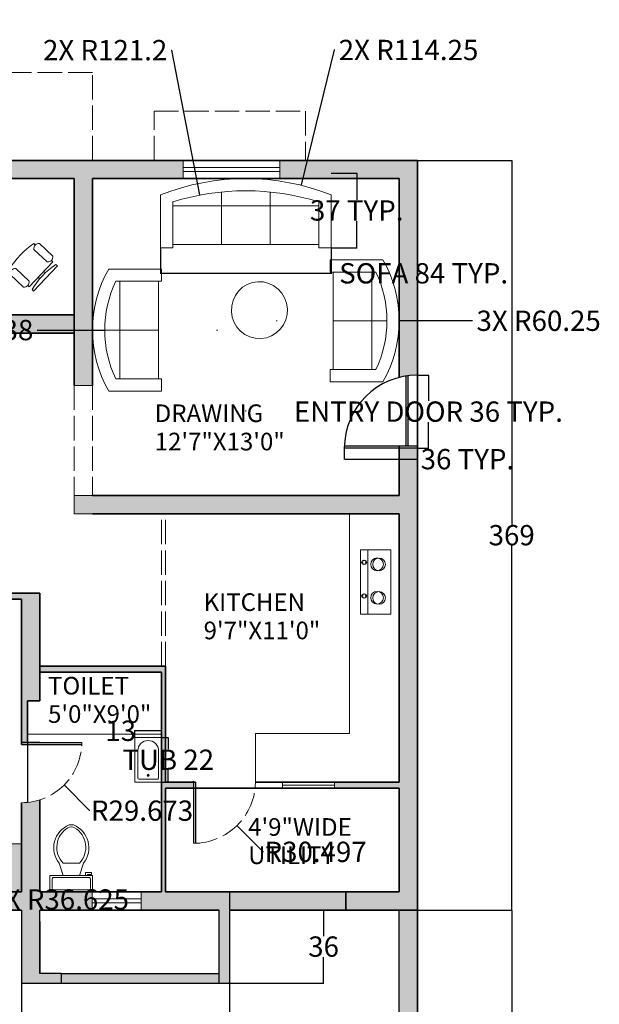
# Model space of a CAD drawing. Units: inches. Extents: x 215 to 969, y -612 to 418.
# Tile 8 of 8: x 684 to 969, y -93 to 391. Entities that reach past the tile are written whole.
import ezdxf

# ---------------------------------------------------------------- set-up
doc = ezdxf.new("R2010")
doc.units = ezdxf.units.IN
doc.header["$MEASUREMENT"] = 0
doc.linetypes.add('ACAD_ISO02W100', pattern=[15, 12, -3])
for name, color, linetype, lineweight in [('A-ANNO-DIMS', 2, 'Continuous', 18), ('A-AREA-IDEN', 7, 'Continuous', 18), ('A-DOOR', 3, 'Continuous', 25), ('A-DOOR-SWNG', 3, 'ACAD_ISO02W100', 13), ('A-EQPM', 8, 'Continuous', 18), ('A-FLOR-CASE', 9, 'Continuous', 18), ('A-FLOR-FIXT', 9, 'Continuous', 18), ('A-FLOR-OVHD', 8, 'ACAD_ISO02W100', 13), ('A-FLOR-SLAB', 7, 'Continuous', 25), ('A-FURN', 8, 'Continuous', 18), ('A-GLAZ', 4, 'Continuous', 18), ('A-WALL', 7, 'Continuous', 35), ('A-WALL-OVHD', 7, 'ACAD_ISO02W100', 18)]:
    doc.layers.add(name, color=color, linetype=linetype, lineweight=lineweight)
doc.layers.add('A-WALL-PATT', color=252, linetype='Continuous', lineweight=13, true_color=0x939598)
doc.styles.get("Standard").update_dxf_attribs({"font": 'arial.ttf'})
doc.dimstyles.get("Standard").update_dxf_attribs({"dimtxt": 10, "dimasz": 0.18, "dimexe": 0.18, "dimexo": 0.0625, "dimgap": 0.09, "dimtad": 0, "dimtih": 1, "dimtoh": 1, "dimdec": 0, "dimzin": 0, "dimdsep": 46, "dimlunit": 3, "dimtxsty": 'Standard', "dimcen": 0.09, "dimadec": 0, "dimazin": 0, "dimtfac": 1, "dimtdec": 0, "dimtofl": 0, "dimtmove": 0, "dimatfit": 3, "dimfxl": 1, "dimtolj": 1, "dimtzin": 0, "dimarcsym": 0})

# ---------------------------------------------------------------- blocks, each defined once
blk = doc.blocks.new('Sofa - Roundback 7 ft.')
for p, q in [((-12.00002, -32.4421), (-12.00003, -6.5971)), ((11.99997, -32.4421), (11.99998, -6.5971)), ((-36.000027, -34), (-36.000027, -11.4696)), ((-35.999844, -13.3819), (35.9998, -13.3819)), ((35.99998, -34), (35.99998, -11.4696)), ((-36.000027, -32.4421), (35.99998, -32.4421))]:
    blk.add_line(p, q)
for points in [[(-36.000027, -34), (-42.000027, -34), (-42.000027, -8)], [(41.99998, -8), (41.99998, -34), (35.99998, -34)]]:
    blk.add_lwpolyline(points)
for centre, radius, start, end in [((0, -114.25), 114.25, 68.43141, 111.5686), ((-0.00001, -127.1968), 121.1968, 72.72033, 107.2797)]:
    blk.add_arc(centre, radius, start, end)
blk = doc.blocks.new('Sofa - Roundback Loveseat 5 ft.')
for p, q in [((0, -32.44198), (0, -5.99998)), ((-24, -33.99998), (-24, -11.46958)), ((-23.9998, -13.38178), (23.99986, -13.38178)), ((24.00004, -33.99998), (24.00004, -11.46958)), ((-24, -32.44198), (24.00004, -32.44198))]:
    blk.add_line(p, q)
for points in [[(-24, -33.99998), (-30, -33.99998), (-30, -7.99998)], [(30.00004, -7.99998), (30.00004, -33.99998), (24.00004, -33.99998)]]:
    blk.add_lwpolyline(points)
for centre, radius, start, end in [((0, -60.24998), 60.24998, 60.13715, 119.8628), ((0, -61.38438), 55.38444, 64.32083, 115.6792)]:
    blk.add_arc(centre, radius, start, end)
blk = doc.blocks.new('Toilet - top')
for p, q in [((9.5, -6), (9.5, -2)), ((-10, -8.5), (-8, -8.5)), ((-10, -9.5), (-10, -8.5)), ((-7, -9.5), (-10, -9.5)), ((-8, -8.5), (-8, -8)), ((-7, -8), (-7, -9.5)), ((-4, -8), (-6, -14)), ((4, -8), (6, -14)), ((4, -14), (-4, -14))]:
    blk.add_line(p, q)
blk.add_lwpolyline([(10.5, -8), (10.5, 0), (-10.5, 0), (-10.5, -8)], close=True)
for points in [[(-9.5, -2), (-9.5, -6)], [(8.5, -1), (-8.5, -1)], [(-8.5, -7), (8.5, -7)]]:
    blk.add_lwpolyline(points)
for centre, radius, start, end in [((-8.62, -1.88), 0.884, 81.8699, 188.1301), ((8.62, -1.88), 0.884, 351.8699, 98.1301), ((-8.62, -6.12), 0.884, 171.8699, 278.1301), ((8.62, -6.12), 0.884, 261.8699, 8.1301), ((3.52, -21.58), 12.17, 141.4691, 247.9714), ((4.2, -21.82), 11.33, 136.3677, 238.9468), ((-3.52, -21.58), 12.17, 292.0284, 38.5307), ((-4.2, -21.82), 11.33, 301.053, 43.6321), ((0, -27.88), 4, 245.7318, 294.2682), ((0, -29), 4, 254.8605, 285.1395)]:
    blk.add_arc(centre, radius, start, end)
blk = doc.blocks.new('Bath Tub - 26 x 60 in.')
for p, q in [((8, -18), (10, -18)), ((9, -17), (9, -19))]:
    blk.add_line(p, q)
blk.add_lwpolyline([(0, -36), (0, 0), (60, 0), (60, -36)], close=True)
for points in [[(4, -30), (4, -6)], [(6, -4), (42, -4)], [(42, -32), (6, -32)]]:
    blk.add_lwpolyline(points)
for radius in [1.5, 1]:
    blk.add_circle((9, -18), radius)
for centre, radius, start, end in [((5.75, -5.75), 1.77, 81.8699, 188.1301), ((42, -18), 14, 270, 90), ((5.75, -30.25), 1.77, 171.8699, 278.1301)]:
    blk.add_arc(centre, radius, start, end)
blk = doc.blocks.new('Chair - Desk')
for p, q in [((-8.5, 0), (-8.5, -1)), ((-8.5, 0), (8.5, 0)), ((8.5, 0), (8.5, -1)), ((-8.5, -3), (-8.5, -4)), ((-8.5, -3), (8.5, -3)), ((-2, -3), (-2, -1.9355)), ((2, -1.9576), (2, -3)), ((8.5, -3), (8.5, -4)), ((-10.5, -5), (-10.5, -14)), ((-6.5, -14), (-6.5, -5)), ((6.5, -5), (6.5, -14)), ((10.5, -14), (10.5, -5)), ((-8.5, -15), (-8.5, -16)), ((8.5, -15), (8.5, -16))]:
    blk.add_line(p, q)
for centre, radius, start, end in [((-8.5, -6.5), 2.5, 36.8699, 143.1301), ((0, 34.625), 36.625, 256.5803, 283.4197), ((8.5, -6.5), 2.5, 36.8699, 143.1301), ((-8.5, -12.5), 2.5, 216.8699, 323.1301), ((8.5, -12.5), 2.5, 216.8699, 323.1301), ((0, 19.625), 36.625, 256.5803, 283.4197)]:
    blk.add_arc(centre, radius, start, end)
blk = doc.blocks.new('WINDOW-SHADE-75')
for p, q in [((0, 0), (0, 24.15)), ((0, 24.15), (74.66, 24.15)), ((74.66, 24.15), (74.66, 0))]:
    blk.add_line(p, q)
blk = doc.blocks.new('DOOR-ENTRY-36')
for p, q in [((36, 1), (0, 1)), ((36, 0), (0, 0))]:
    blk.add_line(p, q)
blk.add_arc((36, 0), 36, 90, 180)
blk = doc.blocks.new('WIN-FRAME-24B')
for p, q in [((0, 23.99), (9, 23.99)), ((3.5, 23.99), (3.5, 0)), ((5.5, 23.99), (5.5, 0)), ((9, 0), (0, 0)), ((4.5, 0), (9, 0))]:
    blk.add_line(p, q)
blk = doc.blocks.new('*D27')
at = {"layer": 'A-ANNO-DIMS', "color": 0, "lineweight": -2, "transparency": 16777216}
for p, q in [((753.42, 38.14), (756.82, 38.14)), ((756.64, 37.96), (756.64, 32.37)), ((756.64, 16.39), (756.64, 21.98)), ((753.42, 16.21), (756.82, 16.21))]:
    blk.add_line(p, q, dxfattribs=at)
at = {"layer": 'A-ANNO-DIMS', "color": 0, "transparency": 16777216}
for points in [[(756.61, 37.96), (756.67, 37.96), (756.64, 38.14)], [(756.61, 16.39), (756.67, 16.39), (756.64, 16.21)]]:
    blk.add_solid(points, dxfattribs=at)
at = {"layer": 'Defpoints', "color": 0, "transparency": 16777216}
for p in [(753.35, 38.14), (756.64, 38.14), (753.35, 16.21)]:
    blk.add_point(p, dxfattribs=at)
at = {"layer": 'A-ANNO-DIMS', "color": 0, "transparency": 16777216, "insert": (756.64, 27.18), "char_height": 10, "attachment_point": 5}
blk.add_mtext('\\A1;TUB 22', dxfattribs=at)
blk = doc.blocks.new('*D28')
at = {"layer": 'A-ANNO-DIMS', "color": 0, "lineweight": -2, "transparency": 16777216}
for p, q in [((740.2, 41.43), (740.02, 41.43)), ((740.2, 38.2), (740.2, 41.61)), ((753.17, 41.43), (740.38, 41.43)), ((753.35, 38.2), (753.35, 41.61))]:
    blk.add_line(p, q, dxfattribs=at)
at = {"layer": 'A-ANNO-DIMS', "color": 0, "transparency": 16777216}
for points in [[(740.38, 41.46), (740.38, 41.4), (740.2, 41.43)], [(753.17, 41.46), (753.17, 41.4), (753.35, 41.43)]]:
    blk.add_solid(points, dxfattribs=at)
at = {"layer": 'Defpoints', "color": 0, "transparency": 16777216}
for p in [(740.2, 41.43), (740.2, 38.14), (753.35, 38.14)]:
    blk.add_point(p, dxfattribs=at)
at = {"layer": 'A-ANNO-DIMS', "color": 0, "transparency": 16777216, "insert": (733.24, 41.43), "char_height": 10, "attachment_point": 5}
blk.add_mtext('\\A1;13', dxfattribs=at)
blk = doc.blocks.new('*D53')
at = {"layer": 'A-ANNO-DIMS', "color": 0, "lineweight": -2, "transparency": 16777216}
for p, q in [((752.85, 279.15), (752.85, 266.43)), ((836.85, 279.15), (836.85, 266.43)), ((753.03, 266.61), (836.67, 266.61)), ((836.85, 266.61), (837.03, 266.61))]:
    blk.add_line(p, q, dxfattribs=at)
at = {"layer": 'A-ANNO-DIMS', "color": 0, "transparency": 16777216}
for points in [[(753.03, 266.64), (753.03, 266.58), (752.85, 266.61)], [(836.67, 266.64), (836.67, 266.58), (836.85, 266.61)]]:
    blk.add_solid(points, dxfattribs=at)
at = {"layer": 'Defpoints', "color": 0, "transparency": 16777216}
for p in [(752.85, 279.21), (836.85, 279.21), (836.85, 266.61)]:
    blk.add_point(p, dxfattribs=at)
at = {"layer": 'A-ANNO-DIMS', "color": 0, "transparency": 16777216, "insert": (882.4, 266.61), "char_height": 10, "attachment_point": 5}
blk.add_mtext('\\A1;SOFA 84 TYP.', dxfattribs=at)
blk = doc.blocks.new('*D54')
at = {"layer": 'A-ANNO-DIMS', "color": 0, "lineweight": -2, "transparency": 16777216}
for p, q in [((836.92, 315.88), (849.63, 315.88)), ((849.45, 315.7), (849.45, 302.75)), ((849.45, 279.39), (849.45, 292.35)), ((836.92, 279.21), (849.63, 279.21))]:
    blk.add_line(p, q, dxfattribs=at)
at = {"layer": 'A-ANNO-DIMS', "color": 0, "transparency": 16777216}
for points in [[(849.42, 315.7), (849.48, 315.7), (849.45, 315.88)], [(849.42, 279.39), (849.48, 279.39), (849.45, 279.21)]]:
    blk.add_solid(points, dxfattribs=at)
at = {"layer": 'Defpoints', "color": 0, "transparency": 16777216}
for p in [(836.85, 315.88), (849.45, 315.88), (836.85, 279.21)]:
    blk.add_point(p, dxfattribs=at)
at = {"layer": 'A-ANNO-DIMS', "color": 0, "transparency": 16777216, "insert": (849.45, 297.55), "char_height": 10, "attachment_point": 5}
blk.add_mtext('\\A1;37 TYP.', dxfattribs=at)
blk = doc.blocks.new('*D63')
at = {"layer": 'A-ANNO-DIMS', "color": 0, "lineweight": -2, "transparency": 16777216}
for p, q in [((879.42, 216.53), (884.93, 216.53)), ((884.75, 216.35), (884.75, 203.8)), ((884.75, 180.71), (884.75, 193.27)), ((879.42, 180.53), (884.93, 180.53))]:
    blk.add_line(p, q, dxfattribs=at)
at = {"layer": 'A-ANNO-DIMS', "color": 0, "transparency": 16777216}
for points in [[(884.72, 216.35), (884.78, 216.35), (884.75, 216.53)], [(884.72, 180.71), (884.78, 180.71), (884.75, 180.53)]]:
    blk.add_solid(points, dxfattribs=at)
at = {"layer": 'Defpoints', "color": 0, "transparency": 16777216}
for p in [(879.35, 216.53), (884.75, 216.53), (879.35, 180.53)]:
    blk.add_point(p, dxfattribs=at)
at = {"layer": 'A-ANNO-DIMS', "color": 0, "transparency": 16777216, "insert": (884.75, 198.53), "char_height": 10, "attachment_point": 5}
blk.add_mtext('\\A1;ENTRY DOOR 36 TYP.', dxfattribs=at)
blk = doc.blocks.new('*D64')
at = {"layer": 'A-ANNO-DIMS', "color": 0, "lineweight": -2, "transparency": 16777216}
for p, q in [((843.35, 180.47), (843.35, 174.95)), ((879.35, 180.47), (879.35, 174.95)), ((843.53, 175.13), (879.17, 175.13)), ((879.35, 175.13), (879.53, 175.13))]:
    blk.add_line(p, q, dxfattribs=at)
at = {"layer": 'A-ANNO-DIMS', "color": 0, "transparency": 16777216}
for points in [[(843.53, 175.16), (843.53, 175.1), (843.35, 175.13)], [(879.17, 175.16), (879.17, 175.1), (879.35, 175.13)]]:
    blk.add_solid(points, dxfattribs=at)
at = {"layer": 'Defpoints', "color": 0, "transparency": 16777216}
for p in [(843.35, 180.53), (879.35, 180.53), (879.35, 175.13)]:
    blk.add_point(p, dxfattribs=at)
at = {"layer": 'A-ANNO-DIMS', "color": 0, "transparency": 16777216, "insert": (903.96, 175.13), "char_height": 10, "attachment_point": 5}
blk.add_mtext('\\A1;36 TYP.', dxfattribs=at)
blk = doc.blocks.new('*D70')
at = {"layer": 'A-ANNO-DIMS', "color": 0, "lineweight": -2, "transparency": 16777216}
for p, q in [((879.42, 322.21), (925.93, 322.21)), ((925.75, 322.03), (925.75, 142.91)), ((925.75, -46.61), (925.75, 132.51)), ((879.42, -46.79), (925.93, -46.79))]:
    blk.add_line(p, q, dxfattribs=at)
at = {"layer": 'A-ANNO-DIMS', "color": 0, "transparency": 16777216}
for points in [[(925.72, 322.03), (925.78, 322.03), (925.75, 322.21)], [(925.72, -46.61), (925.78, -46.61), (925.75, -46.79)]]:
    blk.add_solid(points, dxfattribs=at)
at = {"layer": 'Defpoints', "color": 0, "transparency": 16777216}
for p in [(879.35, 322.21), (879.35, -46.79), (925.75, -46.79)]:
    blk.add_point(p, dxfattribs=at)
at = {"layer": 'A-ANNO-DIMS', "color": 0, "transparency": 16777216, "insert": (925.75, 137.71), "char_height": 10, "attachment_point": 5}
blk.add_mtext('\\A1;369', dxfattribs=at)
blk = doc.blocks.new('*D71')
at = {"layer": 'A-ANNO-DIMS', "color": 0, "lineweight": -2, "transparency": 16777216}
for p, q in [((879.42, -46.79), (925.93, -46.79)), ((925.75, -46.97), (925.75, -101.42)), ((925.75, -166.27), (925.75, -111.82)), ((879.42, -166.45), (925.93, -166.45))]:
    blk.add_line(p, q, dxfattribs=at)
at = {"layer": 'A-ANNO-DIMS', "color": 0, "transparency": 16777216}
for points in [[(925.72, -46.97), (925.78, -46.97), (925.75, -46.79)], [(925.72, -166.27), (925.78, -166.27), (925.75, -166.45)]]:
    blk.add_solid(points, dxfattribs=at)
at = {"layer": 'Defpoints', "color": 0, "transparency": 16777216}
for p in [(879.35, -46.79), (879.35, -166.45), (925.75, -166.45)]:
    blk.add_point(p, dxfattribs=at)
at = {"layer": 'A-ANNO-DIMS', "color": 0, "transparency": 16777216, "insert": (925.75, -106.62), "char_height": 10, "attachment_point": 5}
blk.add_mtext('\\A1;119.67', dxfattribs=at)
blk = doc.blocks.new('*D75')
at = {"layer": 'A-ANNO-DIMS', "color": 0, "lineweight": -2, "transparency": 16777216}
for p, q in [((290.35, 103.15), (290.35, -605.89)), ((879.35, -534.51), (879.35, -605.89)), ((290.53, -605.71), (573.71, -605.71)), ((879.17, -605.71), (596, -605.71))]:
    blk.add_line(p, q, dxfattribs=at)
at = {"layer": 'A-ANNO-DIMS', "color": 0, "transparency": 16777216}
for points in [[(290.53, -605.68), (290.53, -605.74), (290.35, -605.71)], [(879.17, -605.68), (879.17, -605.74), (879.35, -605.71)]]:
    blk.add_solid(points, dxfattribs=at)
at = {"layer": 'Defpoints', "color": 0, "transparency": 16777216}
for p in [(290.35, 103.21), (879.35, -534.45), (879.35, -605.71)]:
    blk.add_point(p, dxfattribs=at)
at = {"layer": 'A-ANNO-DIMS', "color": 0, "transparency": 16777216, "insert": (584.85, -605.71), "char_height": 10, "attachment_point": 5}
blk.add_mtext('\\A1;589', dxfattribs=at)
blk = doc.blocks.new('*D79')
at = {"layer": 'A-ANNO-DIMS', "color": 0, "lineweight": -2, "transparency": 16777216}
for p, q in [((684.35, -82.85), (684.35, -605.89)), ((786.74, -82.85), (786.74, -605.89)), ((684.53, -605.71), (715.16, -605.71)), ((786.56, -605.71), (755.93, -605.71))]:
    blk.add_line(p, q, dxfattribs=at)
at = {"layer": 'A-ANNO-DIMS', "color": 0, "transparency": 16777216}
for points in [[(684.53, -605.68), (684.53, -605.74), (684.35, -605.71)], [(786.56, -605.68), (786.56, -605.74), (786.74, -605.71)]]:
    blk.add_solid(points, dxfattribs=at)
at = {"layer": 'Defpoints', "color": 0, "transparency": 16777216}
for p in [(684.35, -82.79), (786.74, -82.79), (786.74, -605.71)]:
    blk.add_point(p, dxfattribs=at)
at = {"layer": 'A-ANNO-DIMS', "color": 0, "transparency": 16777216, "insert": (735.55, -605.71), "char_height": 10, "attachment_point": 5}
blk.add_mtext('\\A1;102.38', dxfattribs=at)
blk = doc.blocks.new('*D80')
at = {"layer": 'A-ANNO-DIMS', "color": 0, "lineweight": -2, "transparency": 16777216}
for p, q in [((786.8, -46.79), (833.32, -46.79)), ((833.14, -46.97), (833.14, -59.59)), ((833.14, -82.61), (833.14, -69.99)), ((786.8, -82.79), (833.32, -82.79))]:
    blk.add_line(p, q, dxfattribs=at)
at = {"layer": 'A-ANNO-DIMS', "color": 0, "transparency": 16777216}
for points in [[(833.11, -46.97), (833.17, -46.97), (833.14, -46.79)], [(833.11, -82.61), (833.17, -82.61), (833.14, -82.79)]]:
    blk.add_solid(points, dxfattribs=at)
at = {"layer": 'Defpoints', "color": 0, "transparency": 16777216}
for p in [(786.74, -46.79), (786.74, -82.79), (833.14, -82.79)]:
    blk.add_point(p, dxfattribs=at)
at = {"layer": 'A-ANNO-DIMS', "color": 0, "transparency": 16777216, "insert": (833.14, -64.79), "char_height": 10, "attachment_point": 5}
blk.add_mtext('\\A1;36', dxfattribs=at)
blk = doc.blocks.new('*D81')
at = {"layer": 'A-ANNO-DIMS', "color": 0, "lineweight": -2, "transparency": 16777216}
for p, q in [((786.74, -46.85), (786.74, -605.89)), ((879.35, -46.85), (879.35, -605.89)), ((786.92, -605.71), (816.13, -605.71)), ((879.17, -605.71), (849.96, -605.71))]:
    blk.add_line(p, q, dxfattribs=at)
at = {"layer": 'A-ANNO-DIMS', "color": 0, "transparency": 16777216}
for points in [[(786.92, -605.68), (786.92, -605.74), (786.74, -605.71)], [(879.17, -605.68), (879.17, -605.74), (879.35, -605.71)]]:
    blk.add_solid(points, dxfattribs=at)
at = {"layer": 'Defpoints', "color": 0, "transparency": 16777216}
for p in [(786.74, -46.79), (879.35, -46.79), (879.35, -605.71)]:
    blk.add_point(p, dxfattribs=at)
at = {"layer": 'A-ANNO-DIMS', "color": 0, "transparency": 16777216, "insert": (833.05, -605.71), "char_height": 10, "attachment_point": 5}
blk.add_mtext('\\A1;92.62', dxfattribs=at)
blk = doc.blocks.new('*D88')
at = {"layer": 'A-ANNO-DIMS', "color": 0, "lineweight": -2, "transparency": 16777216}
for p, q in [((684.31, 35.71), (684.49, 35.71)), ((684.4, 35.62), (684.4, 35.8)), ((717.94, 2.12), (705.49, 14.59)), ((718.12, 2.12), (717.94, 2.12))]:
    blk.add_line(p, q, dxfattribs=at)
at = {"layer": 'A-ANNO-DIMS', "color": 0, "transparency": 16777216}
blk.add_solid([(705.51, 14.61), (705.47, 14.57), (705.36, 14.72)], dxfattribs=at)
at = {"layer": 'Defpoints', "color": 0, "transparency": 16777216}
for p in [(684.4, 35.71), (705.36, 14.72)]:
    blk.add_point(p, dxfattribs=at)
at = {"layer": 'A-ANNO-DIMS', "color": 0, "transparency": 16777216, "insert": (743.76, 2.12), "char_height": 10, "attachment_point": 5}
blk.add_mtext('\\A1;R29.673', dxfattribs=at)
blk = doc.blocks.new('*D89')
at = {"layer": 'A-ANNO-DIMS', "color": 0, "lineweight": -2, "transparency": 16777216}
for p, q in [((768.99, 16.54), (769.17, 16.54)), ((769.08, 16.45), (769.08, 16.63)), ((803.4, -18.15), (790.66, -5.27)), ((803.58, -18.15), (803.4, -18.15))]:
    blk.add_line(p, q, dxfattribs=at)
at = {"layer": 'A-ANNO-DIMS', "color": 0, "transparency": 16777216}
blk.add_solid([(790.68, -5.25), (790.64, -5.29), (790.53, -5.14)], dxfattribs=at)
at = {"layer": 'Defpoints', "color": 0, "transparency": 16777216}
for p in [(769.08, 16.54), (790.53, -5.14)]:
    blk.add_point(p, dxfattribs=at)
at = {"layer": 'A-ANNO-DIMS', "color": 0, "transparency": 16777216, "insert": (829.21, -18.15), "char_height": 10, "attachment_point": 5}
blk.add_mtext('\\A1;R30.497', dxfattribs=at)
blk = doc.blocks.new('*D90')
at = {"layer": 'A-ANNO-DIMS', "color": 0, "lineweight": -2, "transparency": 16777216}
for p, q in [((758.11, 376.45), (758.29, 376.45)), ((758.29, 376.45), (771.97, 305.22)), ((794.76, 186.02), (794.94, 186.02)), ((794.85, 185.93), (794.85, 186.11))]:
    blk.add_line(p, q, dxfattribs=at)
at = {"layer": 'A-ANNO-DIMS', "color": 0, "transparency": 16777216}
blk.add_solid([(772, 305.22), (771.94, 305.21), (772, 305.04)], dxfattribs=at)
at = {"layer": 'Defpoints', "color": 0, "transparency": 16777216}
for p in [(772, 305.04), (794.85, 186.02)]:
    blk.add_point(p, dxfattribs=at)
at = {"layer": 'A-ANNO-DIMS', "color": 0, "transparency": 16777216, "insert": (725.58, 376.45), "char_height": 10, "attachment_point": 5}
blk.add_mtext('\\A1;2X R121.2', dxfattribs=at)
blk = doc.blocks.new('*D91')
at = {"layer": 'A-ANNO-DIMS', "color": 0, "lineweight": -2, "transparency": 16777216}
for p, q in [((838.29, 376.53), (822.04, 310.12)), ((838.47, 376.53), (838.29, 376.53)), ((794.76, 198.96), (794.94, 198.96)), ((794.85, 198.87), (794.85, 199.05))]:
    blk.add_line(p, q, dxfattribs=at)
at = {"layer": 'A-ANNO-DIMS', "color": 0, "transparency": 16777216}
blk.add_solid([(822.01, 310.12), (822.07, 310.11), (822, 309.94)], dxfattribs=at)
at = {"layer": 'Defpoints', "color": 0, "transparency": 16777216}
for p in [(822, 309.94), (794.85, 198.96)]:
    blk.add_point(p, dxfattribs=at)
at = {"layer": 'A-ANNO-DIMS', "color": 0, "transparency": 16777216, "insert": (874.97, 376.53), "char_height": 10, "attachment_point": 5}
blk.add_mtext('\\A1;2X R114.25', dxfattribs=at)
blk = doc.blocks.new('*D92')
at = {"layer": 'A-ANNO-DIMS', "color": 0, "lineweight": -2, "transparency": 16777216}
for p, q in [((810.01, 243.25), (810.19, 243.25)), ((810.1, 243.16), (810.1, 243.34)), ((906.5, 243.25), (870.53, 243.25))]:
    blk.add_line(p, q, dxfattribs=at)
at = {"layer": 'A-ANNO-DIMS', "color": 0, "transparency": 16777216}
blk.add_solid([(870.53, 243.28), (870.53, 243.22), (870.35, 243.25)], dxfattribs=at)
at = {"layer": 'Defpoints', "color": 0, "transparency": 16777216}
for p in [(810.1, 243.25), (870.35, 243.25)]:
    blk.add_point(p, dxfattribs=at)
at = {"layer": 'A-ANNO-DIMS', "color": 0, "transparency": 16777216, "insert": (939.03, 243.25), "char_height": 10, "attachment_point": 5}
blk.add_mtext('\\A1;3X R60.25', dxfattribs=at)
blk = doc.blocks.new('*D93')
at = {"layer": 'A-ANNO-DIMS', "color": 0, "lineweight": -2, "transparency": 16777216}
for p, q in [((692.12, 238.67), (725.17, 238.67)), ((780.65, 238.67), (780.83, 238.67)), ((780.74, 238.58), (780.74, 238.76))]:
    blk.add_line(p, q, dxfattribs=at)
at = {"layer": 'A-ANNO-DIMS', "color": 0, "transparency": 16777216}
blk.add_solid([(725.17, 238.7), (725.17, 238.64), (725.35, 238.67)], dxfattribs=at)
at = {"layer": 'Defpoints', "color": 0, "transparency": 16777216}
for p in [(725.35, 238.67), (780.74, 238.67)]:
    blk.add_point(p, dxfattribs=at)
at = {"layer": 'A-ANNO-DIMS', "color": 0, "transparency": 16777216, "insert": (659.62, 238.67), "char_height": 10, "attachment_point": 5}
blk.add_mtext('\\A1;3X R55.38', dxfattribs=at)
blk = doc.blocks.new('*D94')
at = {"layer": 'A-ANNO-DIMS', "color": 0, "lineweight": -2, "transparency": 16777216}
for p, q in [((659.08, 17.02), (659.26, 17.02)), ((659.17, 16.93), (659.17, 17.11)), ((659.17, -41.58), (659.17, -19.78)), ((659.35, -41.58), (659.17, -41.58))]:
    blk.add_line(p, q, dxfattribs=at)
at = {"layer": 'A-ANNO-DIMS', "color": 0, "transparency": 16777216}
blk.add_solid([(659.2, -19.78), (659.14, -19.78), (659.17, -19.6)], dxfattribs=at)
at = {"layer": 'Defpoints', "color": 0, "transparency": 16777216}
for p in [(659.17, 17.02), (659.17, -19.6)]:
    blk.add_point(p, dxfattribs=at)
at = {"layer": 'A-ANNO-DIMS', "color": 0, "transparency": 16777216, "insert": (699.18, -41.58), "char_height": 10, "attachment_point": 5}
blk.add_mtext('\\A1;14X R36.625', dxfattribs=at)

msp = doc.modelspace()

# ---------------------------------------------------------------- hatches: boundary and pattern name
at = {"layer": 'A-WALL-PATT'}
h = msp.add_hatch(color=256, dxfattribs=at)
h.dxf.hatch_style = 1
h.paths.add_polyline_path([(764.0736, 322.2135), (569.3535, 322.2135), (565.0643, 322.2135), (565.0643, 313.2135), (569.3535, 313.2135), (569.3535, 205.2135), (509.3535, 205.2135), (509.3535, 247.2592), (506.3535, 247.2592), (506.3535, 172.2135), (491.3535, 172.2135), (491.3535, 169.2135), (509.3535, 169.2135), (509.3535, 202.2135), (569.3535, 202.2135), (569.3535, 169.2135), (578.3535, 169.2135), (578.3535, 205.2135), (578.3535, 237.2135), (615.7789, 237.2135), (615.7789, 246.2135), (578.3535, 246.2135), (578.3535, 313.2135), (710.3535, 313.2135), (710.3535, 246.2135), (710.3535, 211.3874), (719.3535, 211.3874), (719.3535, 295.2135), (719.3535, 313.2135), (764.0736, 313.2135)])
h.paths.add_polyline_path([(879.3535, 322.2135), (811.6486, 322.2135), (811.6486, 313.2135), (870.3535, 313.2135), (870.3535, 215.3905, -0.06325422), (879.3535, 216.5337), (879.3535, 313.2135)])
h.paths.add_polyline_path([(879.3535, 157.2135), (879.3535, 180.5337), (870.3535, 180.5337), (870.3535, 157.2135), (719.3535, 157.2135), (710.3535, 157.2135), (710.3535, 148.2135), (719.3535, 148.2135), (870.3535, 148.2135), (870.3535, 16.2135), (838.4933, 16.2135), (838.4933, 13.2135), (870.3535, 13.2135), (870.3535, -37.7865), (844.0345, -37.7865), (844.0345, -46.7865), (870.3535, -46.7865), (879.3535, -46.7865), (879.3535, -37.7865), (879.3535, 137.613)])
h.paths.add_polyline_path([(710.3535, 246.2135), (663.4146, 246.2135), (663.4146, 237.2135), (710.3535, 237.2135)], flags=17)
h.paths.add_polyline_path([(541.2942, 322.2135), (509.3535, 322.2135), (468.3222, 322.2135), (468.3222, 313.2135), (500.3535, 313.2135), (509.3535, 313.2135), (541.2942, 313.2135)])
h.paths.add_polyline_path([(509.3535, 313.2135), (503.3535, 313.2135), (503.3535, 277.5241, -0.04952579), (509.3535, 277.4203)], flags=17)
h.paths.add_polyline_path([(420.2828, 322.2135), (335.3535, 322.2135), (335.3535, 235.2487), (344.3535, 235.2487), (344.3535, 284.1885), (344.3535, 313.2135), (420.2828, 313.2135)])
h.paths.add_polyline_path([(335.3535, 181.2135), (290.3535, 181.2135), (290.3535, 103.2135), (335.3535, 103.2135), (335.3535, 112.2135), (299.3535, 112.2135), (299.3535, 129.1615), (299.3535, 172.2135), (335.3535, 172.2135)])
h.paths.add_polyline_path([(344.3535, 199.3097), (335.3535, 199.3097), (335.3535, 172.2135), (335.3535, 157.3369), (344.3535, 157.3369), (344.3535, 169.2135), (452.3535, 169.2135), (452.5037, 169.2135), (452.5037, 150.1199), (452.3535, 109.2135), (455.3535, 109.2135), (455.3535, 169.2135, -0.02086055), (455.4787, 172.2135), (344.3535, 172.2135)])
h.paths.add_polyline_path([(344.3535, 133.3441), (335.3535, 133.3441), (335.3535, 77.89), (344.3535, 77.89), (344.3535, 103.2135), (401.3556, 103.2135), (401.3556, 109.2135), (344.3535, 109.2135)])
h.paths.add_polyline_path([(462.6362, 109.2135), (443.0437, 109.2135), (425.2018, 109.2135), (425.2018, 106.2135), (452.3535, 106.2135), (462.7615, 106.2135, -0.02086055)])
h.paths.add_polyline_path([(540.3535, 106.2135), (684.3535, 106.2135), (684.3535, 35.7135), (687.3535, 35.7135), (687.3535, 56.1856), (693.3535, 56.1856), (693.3535, 109.2135), (540.3535, 109.2135), (531.3535, 109.2135), (498.6362, 109.2135), (498.6362, 106.2135), (531.3535, 106.2135), (531.3535, -37.7865), (507.9524, -37.7865), (507.9524, -46.7865), (610.6038, -46.7865), (610.6038, -37.7865), (540.3535, -37.7865)])
h.paths.add_polyline_path([(578.3535, 358.6622), (555.879, 358.6622), (555.879, 349.6622), (569.3535, 349.6622), (569.3535, 322.2135), (578.3535, 322.2135)])
h.paths.add_polyline_path([(525.962, 358.6622), (503.3535, 358.6622), (503.3535, 322.2135), (509.3535, 322.2135), (509.3535, 349.6622), (525.962, 349.6622)])
h.paths.add_polyline_path([(344.3535, 30.022), (335.3535, 30.022), (335.3535, -37.7865), (335.3535, -46.7865), (484.3302, -46.7865), (484.3302, -37.7865), (344.3535, -37.7865)])
h.paths.add_polyline_path([(719.1188, -37.7865), (698.4193, -37.7865), (693.3535, -37.7865), (693.3535, 7.424, -0.07717369), (684.3535, 6.0404), (684.3535, -37.7865), (658.8269, -37.7865), (658.8269, -46.7865), (684.3535, -46.7865), (684.3535, -82.7865), (693.3535, -82.7865), (704.1236, -82.7865), (704.1236, -78.0462), (693.3535, -78.0462), (693.3535, -46.7865), (719.1188, -46.7865)])
h.paths.add_polyline_path([(684.3535, -14.2202), (669.6716, -14.2202), (669.6716, -16.6044, -0.23606798), (667.6716, -17.6044), (667.6716, -18.6044, -0.11764706), (650.6716, -18.6044), (650.6716, -17.6044, -0.23606798), (648.6716, -16.6044), (648.6716, -14.2202), (603.0565, -14.2202), (603.0565, -37.7865), (684.3535, -37.7865)], flags=17)
h.paths.add_polyline_path([(665.6716, -14.2202), (652.6716, -14.2202), (652.6716, -16.6044, -0.23606798), (650.6716, -17.6044), (650.6716, -18.6044, 0.11764706), (667.6716, -18.6044), (667.6716, -17.6044, -0.23606798), (665.6716, -16.6044)], flags=16)
h.paths.add_polyline_path([(786.7385, -37.7865), (755.3535, -37.7865), (755.3535, 13.2135), (769.0808, 13.2135), (769.0808, 16.2135), (755.3535, 16.2135), (755.3535, 73.2135), (753.3535, 73.2135), (693.3535, 73.2135), (693.3535, 70.2135), (753.3535, 70.2135), (753.3535, -37.7865), (743.3062, -37.7865), (743.3062, -46.7865), (781.7385, -46.7865), (781.7385, -82.7865), (786.7385, -82.7865), (786.7385, -82.3744), (786.7385, -46.7865)])
h.paths.add_polyline_path([(844.0345, -37.7865), (786.7385, -37.7865), (786.7385, -46.7865), (844.0345, -46.7865)], flags=17)
h.paths.add_polyline_path([(781.7385, -78.0462), (704.1236, -78.0462), (704.1236, -82.7865), (781.7385, -82.7865)], flags=17)
h.paths.add_polyline_path([(344.3535, -46.7865), (335.3535, -46.7865), (335.3535, -166.4525), (344.3535, -166.4525)])
h.paths.add_polyline_path([(382.6632, 103.2135), (344.3535, 103.2135), (344.3535, 77.89), (344.3535, 32.7135), (363.5083, 32.7135), (382.6632, 32.7135)])
h.paths.add_polyline_path([(879.3535, -46.7865), (870.3535, -46.7865), (870.3535, -166.4525), (879.3535, -166.4525)])
h.paths.add_polyline_path([(879.3535, -166.4525), (799.4745, -166.4525), (799.4745, -175.4525), (855.3535, -175.4525), (870.3535, -175.4525), (870.3535, -192.5449), (879.3535, -192.5449), (879.3535, -175.4525)])
h.paths.add_polyline_path([(763.1775, -166.4525), (655.7214, -166.4525), (655.7214, -175.4525), (763.1775, -175.4525)])
h.paths.add_polyline_path([(619.8538, -166.4525), (550.8369, -166.4525), (550.8369, -175.4525), (619.8538, -175.4525)])
h.paths.add_polyline_path([(527.1282, -166.4525), (427.0819, -166.4525), (427.0819, -175.4525), (527.1282, -175.4525)])
h.paths.add_polyline_path([(391.4021, -166.4525), (335.3535, -166.4525), (335.3535, -175.4525), (335.3535, -236.0109), (344.3535, -236.0109), (344.3535, -187.5037), (344.3535, -175.4525), (391.4021, -175.4525)])
h.paths.add_polyline_path([(344.3535, -271.9249), (335.3535, -271.9249), (335.3535, -331.0209), (344.3535, -331.0209), (344.3535, -314.4525), (412.4218, -314.4525, -0.02503209), (412.3073, -311.4525), (344.3535, -311.4525)])
h.paths.add_polyline_path([(470.1954, -311.4525), (442.3073, -311.4525), (442.3073, -314.4525), (470.0702, -314.4525, -0.02086055)])
h.paths.add_polyline_path([(455.3535, -314.4525), (452.3535, -314.4525), (452.3535, -374.4525), (455.3535, -374.4525)])
h.paths.add_polyline_path([(579.3535, -241.4072), (519.3535, -241.4072), (519.3535, -283.4525), (579.3535, -283.4525)])
h.paths.add_polyline_path([(516.5043, -281.1089), (584.3098, -281.1089), (584.3098, -264.0138), (516.5043, -264.0138)], flags=9)
h.paths.add_polyline_path([(516.4662, -263.2183), (581.1504, -263.2183), (581.1504, -245.8948), (516.4662, -245.8948)], flags=9)

# ---------------------------------------------------------------- linework, layer by layer
at = {"layer": 'A-DOOR'}
for p, q in [((873.8535, 181.5337), (873.8535, 216.1111)), ((874.8535, 181.5337), (874.8535, 216.2513)), ((693.3535, 35.7135), (684.3535, 35.7135)), ((684.3535, 35.7135), (714.0714, 35.7135)), ((684.3535, 35.7135), (684.3535, 34.7135)), ((684.3535, 34.7135), (714.0714, 34.7135)), ((687.3535, 35.7135), (687.3535, 6.1879)), ((769.0808, 16.2135), (769.0808, -13.9592)), ((770.0808, 16.2135), (770.0808, -13.9592))]:
    msp.add_line(p, q, dxfattribs=at)
at = {"layer": 'A-DOOR-SWNG'}
for centre, radius, start, end in [((684.3982, 35.7135), 29.6732, 269.913661, 0), ((769.0808, 16.5373), 30.4965, 270, 359.391648)]:
    msp.add_arc(centre, radius, start, end, dxfattribs=at)
at = {"layer": 'A-EQPM'}
for p, q in [((854.8726, 130.5735), (854.8726, 129.2287)), ((854.8726, 129.2287), (854.8726, 98.9045))]:
    msp.add_line(p, q, dxfattribs=at)
msp.add_lwpolyline([(851.3651, 130.5735), (866.243, 130.5735), (866.243, 98.9045), (851.3651, 98.9045)], close=True, dxfattribs=at)
for centre, radius in [((859.472, 123.3688), 3.1316), ((860.4391, 123.3152), 3.1316), ((852.8878, 124.3693), 1.0177), ((853.3407, 124.3693), 1.0177), ((852.8878, 107.7702), 1.0177), ((853.3407, 107.7702), 1.0177), ((859.472, 106.9064), 3.1316), ((860.4391, 106.8528), 3.1316)]:
    msp.add_circle(centre, radius, dxfattribs=at)
at = {"layer": 'A-FLOR-CASE'}
for p, q in [((870.3535, 148.2135), (845.8922, 148.2135)), ((845.8922, 148.2135), (845.8922, 40.0988)), ((845.8922, 40.0988), (799.5756, 40.0988)), ((799.5756, 40.0988), (799.5756, 16.2135)), ((684.3535, -14.2202), (540.3535, -14.2202))]:
    msp.add_line(p, q, dxfattribs=at)
at = {"layer": 'A-FLOR-FIXT'}
msp.add_line((687.3535, 39.8514), (753.3535, 39.8514), dxfattribs=at)
at = {"layer": 'A-FLOR-OVHD'}
for p, q in [((719.3535, 365.5008), (569.3535, 365.5008)), ((719.3535, 322.2135), (719.3535, 365.5008))]:
    msp.add_line(p, q, dxfattribs=at)
at = {"layer": 'A-FLOR-SLAB'}
for p, q in [((786.7385, -37.7865), (786.7385, -46.7865)), ((684.3535, -46.7865), (684.3535, -82.7865)), ((693.3535, -78.0462), (693.3535, -46.7865)), ((781.7385, -82.7865), (781.7385, -46.7865)), ((786.7385, -46.7865), (786.7385, -82.3744)), ((870.3535, -166.4525), (870.3535, -46.7865)), ((879.3535, -175.4525), (879.3535, -46.7865)), ((693.3535, -52.4202), (693.3535, -78.0462)), ((704.1236, -78.0462), (693.3535, -78.0462)), ((704.1236, -82.7865), (704.1236, -78.0462)), ((704.1236, -78.0462), (781.7385, -78.0462)), ((786.7385, -82.7865), (786.7385, -82.3744)), ((684.3535, -82.7865), (693.3535, -82.7865)), ((693.3535, -82.7865), (704.1236, -82.7865)), ((704.1236, -82.7865), (786.7385, -82.7865))]:
    msp.add_line(p, q, dxfattribs=at)
at = {"layer": 'A-FURN'}
msp.add_ellipse((801.5426, 248.4784), major_axis=(0.7087, -14.0145), ratio=0.98393012, dxfattribs=at)
at = {"layer": 'A-GLAZ'}
for p, q in [((764.0736, 322.2135), (764.0736, 313.2135)), ((811.6486, 317.7135), (811.6486, 322.2135)), ((811.6486, 322.2135), (811.6486, 313.2135)), ((764.0736, 318.7135), (811.6486, 318.7135)), ((764.0736, 316.7135), (811.6486, 316.7135)), ((812.8535, 16.2135), (812.8535, 13.2135)), ((812.8535, 14.7135), (838.4933, 14.7135)), ((838.4933, 16.2135), (838.4933, 13.2135))]:
    msp.add_line(p, q, dxfattribs=at)
at = {"layer": 'A-WALL'}
for p, q in [((569.3535, 322.2135), (879.3535, 322.2135)), ((578.3535, 322.2135), (710.3535, 322.2135)), ((719.3535, 322.2135), (870.3535, 322.2135)), ((879.3535, 322.2135), (879.3535, 313.2135)), ((578.3535, 313.2135), (710.3535, 313.2135)), ((710.3535, 313.2135), (710.3535, 295.2135)), ((719.3535, 313.2135), (719.3535, 295.2135)), ((719.3535, 313.2135), (870.3535, 313.2135)), ((870.3535, 313.2135), (870.3535, 215.3905)), ((879.3535, 313.2135), (879.3535, 157.2135)), ((710.3535, 295.2135), (710.3535, 211.3874)), ((719.3535, 295.2135), (719.3535, 211.3874)), ((710.3535, 246.2135), (578.3535, 246.2135)), ((710.3535, 237.2135), (578.3535, 237.2135)), ((870.3535, 181.5337), (870.3535, 157.2135)), ((870.3535, 157.2135), (719.3535, 157.2135)), ((879.3535, 157.2135), (879.3535, 137.613)), ((870.3535, 148.2135), (719.3535, 148.2135)), ((870.3535, 148.2135), (870.3535, 16.2135)), ((879.3535, 148.2135), (879.3535, 16.2135)), ((879.3535, 137.613), (879.3535, -37.7865)), ((540.3535, 109.2135), (693.3535, 109.2135)), ((693.3535, 109.2135), (693.3535, 56.1856)), ((540.3535, 106.2135), (684.3535, 106.2135)), ((684.3535, 106.2135), (684.3535, 34.7135)), ((753.3535, 73.2135), (693.3535, 73.2135)), ((755.3535, 73.2135), (753.3535, 73.2135)), ((755.3535, 16.2135), (755.3535, 73.2135)), ((753.3535, 70.2135), (693.3535, 70.2135)), ((753.3535, -37.7865), (753.3535, 70.2135)), ((687.3535, 35.7135), (687.3535, 56.1856)), ((687.3535, 56.1856), (693.3535, 56.1856)), ((770.0808, 16.2135), (755.3535, 16.2135)), ((870.3535, 16.2135), (799.5756, 16.2135)), ((870.3535, 13.2135), (755.3535, 13.2135)), ((755.3535, -37.7865), (755.3535, 13.2135)), ((870.3535, 13.2135), (870.3535, -37.7865)), ((879.3535, 13.2135), (879.3535, -37.7865)), ((684.3535, 6.0404), (684.3535, -37.7865)), ((693.3535, 7.424), (693.3535, -37.7865)), ((684.3535, -37.7865), (540.3535, -37.7865)), ((693.3535, -37.7865), (753.3535, -37.7865)), ((870.3535, -37.7865), (755.3535, -37.7865)), ((844.0345, -37.7865), (844.0345, -46.7865)), ((879.3535, -37.7865), (879.3535, -46.7865)), ((684.3535, -46.7865), (335.3535, -46.7865)), ((684.3535, -46.7865), (540.3535, -46.7865)), ((693.3535, -46.7865), (753.3535, -46.7865)), ((781.7385, -46.7865), (693.3535, -46.7865)), ((781.7385, -46.7865), (755.3535, -46.7865)), ((870.3535, -46.7865), (786.7385, -46.7865)), ((870.3535, -46.7865), (786.7385, -46.7865)), ((879.3535, -46.7865), (870.3535, -46.7865))]:
    msp.add_line(p, q, dxfattribs=at)
at = {"layer": 'A-WALL-OVHD'}
for p, q in [((710.3535, 313.2135), (710.3535, 313.2135)), ((710.3535, 313.2135), (710.3535, 246.2135)), ((879.3535, 180.5337), (879.3535, 216.5337)), ((719.3535, 211.3874), (710.3535, 211.3874)), ((710.3535, 211.3874), (710.3535, 157.2135)), ((719.3535, 211.3874), (719.3535, 157.2135)), ((870.3535, 180.5337), (879.3535, 180.5337)), ((710.3535, 148.2135), (710.3535, 157.2135)), ((710.3535, 157.2135), (719.3535, 157.2135)), ((719.3535, 148.2135), (710.3535, 148.2135)), ((753.3535, 73.2135), (753.3535, 148.2135)), ((755.3535, 73.2135), (755.3535, 148.2135))]:
    msp.add_line(p, q, dxfattribs=at)

# ---------------------------------------------------------------- block references
at = {"layer": 'A-DOOR'}
msp.add_blockref('DOOR-ENTRY-36', (843.353, 180.534), dxfattribs=at)
at = {"layer": 'A-FLOR-FIXT', "xscale": 0.3654102738436262, "yscale": 0.3654102738436262, "zscale": 0.3654102738436262, "rotation": 90}
msp.add_blockref('Bath Tub - 26 x 60 in.', (740.1987, 16.2135), dxfattribs=at)
at = {"layer": 'A-FLOR-FIXT', "rotation": 180}
msp.add_blockref('Toilet - top', (708.9193, -37.7865), dxfattribs=at)
at = {"layer": 'A-FLOR-OVHD'}
msp.add_blockref('WINDOW-SHADE-75', (749.652, 322.214), dxfattribs=at)
at = {"layer": 'A-FURN'}
msp.add_blockref('Sofa - Roundback 7 ft.', (794.8535, 313.2135), dxfattribs=at)
for name, p, rotation in [('Chair - Desk', (696.2113, 264.0519), 226.5917899333866), ('Sofa - Roundback Loveseat 5 ft.', (870.3535, 243.2462), 270), ('Sofa - Roundback Loveseat 5 ft.', (719.3535, 238.6687), 90)]:
    msp.add_blockref(name, p, dxfattribs=dict(at, rotation=rotation))
at = {"layer": 'A-GLAZ', "extrusion": (0, 0, -1), "yscale": 1.008110169064693, "zscale": -1, "rotation": 90}
msp.add_blockref('WIN-FRAME-24B', (-719.1187, -46.7869), dxfattribs=at)

# ---------------------------------------------------------------- texts
at = {"layer": 'A-AREA-IDEN'}
for s, height, p in [('DRAWING', 8.67737, (749.987, 193.3904)), ('12\'7"X13\'0"', 8.677368, (749.987, 179.451)), ('KITCHEN', 8.67737, (774.0698, 100.4232)), ('9\'7"X11\'0"', 8.67737, (774.0698, 86.4838)), ('TOILET', 8.67737, (697.4607, 59.2836)), ('5\'0"X9\'0"', 8.67737, (697.4607, 45.3442)), ('4\'9"WIDE', 8.67737, (795.9921, -10.2408)), ('UTILITY', 8.67737, (795.9921, -24.1802))]:
    msp.add_text(s, height=height, dxfattribs=at).set_placement(p)

# ---------------------------------------------------------------- dimensions: what is measured, and where the dimension line sits
at = {"layer": 'A-ANNO-DIMS'}
for center, mpoint, text, override, picture, middle in [((794.8535, 186.0168), (772.0001, 305.0394), '2X <>', {"dimdec": 1, "dimlfac": 1, "dimrnd": 0, "dimzin": 0, "dimdsep": 46, "dimlunit": 2}, '*D90', (725.5829, 376.453)), ((794.8535, 198.9635), (822.0004, 309.9415), '2X <>', {"dimdec": 2, "dimlfac": 1, "dimrnd": 0, "dimzin": 0, "dimdsep": 46, "dimlunit": 2}, '*D91', (874.9671, 376.5283)), ((810.1035, 243.2462), (870.3535, 243.246), '3X <>', {"dimdec": 2, "dimlfac": 1, "dimrnd": 0, "dimzin": 0, "dimdsep": 46, "dimlunit": 2}, '*D92', (906.5035, 243.2459)), ((780.7379, 238.6687), (725.3534, 238.669), '3X <>', {"dimdec": 2, "dimlfac": 1, "dimrnd": 0, "dimzin": 0, "dimdsep": 46, "dimlunit": 2}, '*D93', (692.1228, 238.6692)), ((659.1716, 17.0206), (659.172, -19.6044), '14X <>', {"dimdec": 3, "dimlfac": 1, "dimrnd": 0, "dimzin": 0, "dimdsep": 46, "dimlunit": 2}, '*D94', (699.1796, -41.5794))]:
    dim = msp.add_radius_dim(center=center, mpoint=mpoint, text=text, dimstyle='Standard', override=override, dxfattribs=at)
    dim.commit()
    dim.dimension.update_dxf_attribs({"geometry": picture, "text_midpoint": middle, "dimtype": 164})
for base, p1, p2, angle, override, picture, middle in [((925.7535, -46.7865), (879.3535, 322.2135), (879.3535, -46.7865), 90, {"dimdec": 0, "dimlfac": 1, "dimrnd": 0, "dimzin": 0, "dimdsep": 46, "dimlunit": 2}, '*D70', (925.7535, 137.7135)), ((740.1987, 41.4269), (753.3535, 38.1382), (740.1987, 38.1382), 180, {"dimdec": 0, "dimlfac": 1, "dimrnd": 0, "dimzin": 0, "dimdsep": 46, "dimlunit": 2}, '*D28', (733.237, 41.4269)), ((833.1385, -82.7865), (786.7385, -46.7865), (786.7385, -82.7865), 270, {"dimdec": 0, "dimlfac": 1, "dimrnd": 0, "dimzin": 0, "dimdsep": 46, "dimlunit": 2}, '*D80', (833.1385, -64.7865)), ((925.7535, -166.4525), (879.3535, -46.7865), (879.3535, -166.4525), 90, {"dimdec": 2, "dimlfac": 1, "dimrnd": 0, "dimzin": 0, "dimdsep": 46, "dimlunit": 2}, '*D71', (925.7535, -106.6195))]:
    dim = msp.add_linear_dim(base=base, p1=p1, p2=p2, angle=angle, dimstyle='Standard', override=override, dxfattribs=at)
    dim.commit()
    dim.dimension.update_dxf_attribs({"geometry": picture, "text_midpoint": middle})
for base, p1, p2, text, picture, middle in [((849.4535, 315.8802), (836.8535, 279.2135), (836.8535, 315.8802), '<> TYP.', '*D54', (849.4535, 297.5469)), ((884.7535, 216.5337), (879.3535, 180.5337), (879.3535, 216.5337), 'ENTRY DOOR <> TYP.', '*D63', (884.7535, 198.5337)), ((756.6422, 38.1382), (753.3535, 16.2135), (753.3535, 38.1382), 'TUB <>', '*D27', (756.6422, 27.1759))]:
    dim = msp.add_linear_dim(base=base, p1=p1, p2=p2, angle=90, text=text, dimstyle='Standard', override={"dimdec": 0, "dimlfac": 1, "dimrnd": 0, "dimzin": 0, "dimdsep": 46, "dimlunit": 2}, dxfattribs=at)
    dim.commit()
    dim.dimension.update_dxf_attribs({"geometry": picture, "text_midpoint": middle})
for base, p1, p2, text, picture, middle in [((836.8535, 266.6135), (752.8535, 279.2135), (836.8535, 279.2135), 'SOFA <> TYP.', '*D53', (882.3963, 266.6135)), ((879.3535, 175.1337), (843.3535, 180.5337), (879.3535, 180.5337), '<> TYP.', '*D64', (903.9584, 175.1337))]:
    dim = msp.add_linear_dim(base=base, p1=p1, p2=p2, text=text, dimstyle='Standard', override={"dimdec": 0, "dimlfac": 1, "dimrnd": 0, "dimzin": 0, "dimdsep": 46, "dimlunit": 2}, dxfattribs=at)
    dim.commit()
    dim.dimension.update_dxf_attribs({"geometry": picture, "text_midpoint": middle})
for base, p1, p2, override, picture, middle in [((879.3535, -605.7132), (290.3535, 103.2135), (879.3535, -534.4525), {"dimdec": 0, "dimlfac": 1, "dimrnd": 0, "dimzin": 0, "dimdsep": 46, "dimlunit": 2}, '*D75', (584.8535, -605.7132)), ((879.35349, -605.71316), (786.73847, -46.78645), (879.35349, -46.78645), {"dimdec": 2, "dimlfac": 1, "dimrnd": 0, "dimzin": 0, "dimdsep": 46, "dimlunit": 2}, '*D81', (833.04598, -605.71316)), ((786.73847, -605.71316), (684.35349, -82.78645), (786.73847, -82.78645), {"dimdec": 2, "dimlfac": 1, "dimrnd": 0, "dimzin": 0, "dimdsep": 46, "dimlunit": 2}, '*D79', (735.54598, -605.71316))]:
    dim = msp.add_linear_dim(base=base, p1=p1, p2=p2, dimstyle='Standard', override=override, dxfattribs=at)
    dim.commit()
    dim.dimension.update_dxf_attribs({"geometry": picture, "text_midpoint": middle})
for center, mpoint, picture, middle in [((684.3982, 35.7135), (705.3649, 14.7161), '*D88', (743.7573, 2.1176)), ((769.08082, 16.53735), (790.53022, -5.14122), '*D89', (829.21216, -18.14837))]:
    dim = msp.add_radius_dim(center=center, mpoint=mpoint, dimstyle='Standard', override={"dimdec": 3, "dimlfac": 1, "dimrnd": 0, "dimzin": 0, "dimdsep": 46, "dimlunit": 2}, dxfattribs=at)
    dim.commit()
    dim.dimension.update_dxf_attribs({"geometry": picture, "text_midpoint": middle, "dimtype": 164})

doc.saveas('drawing.dxf')
